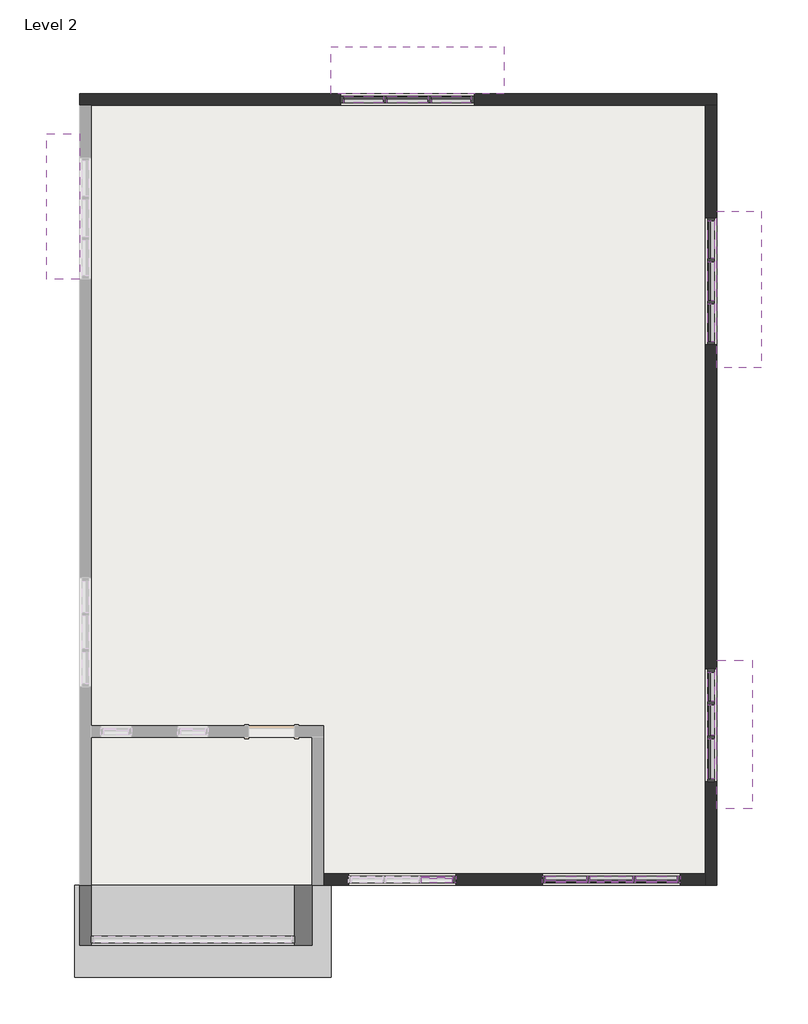
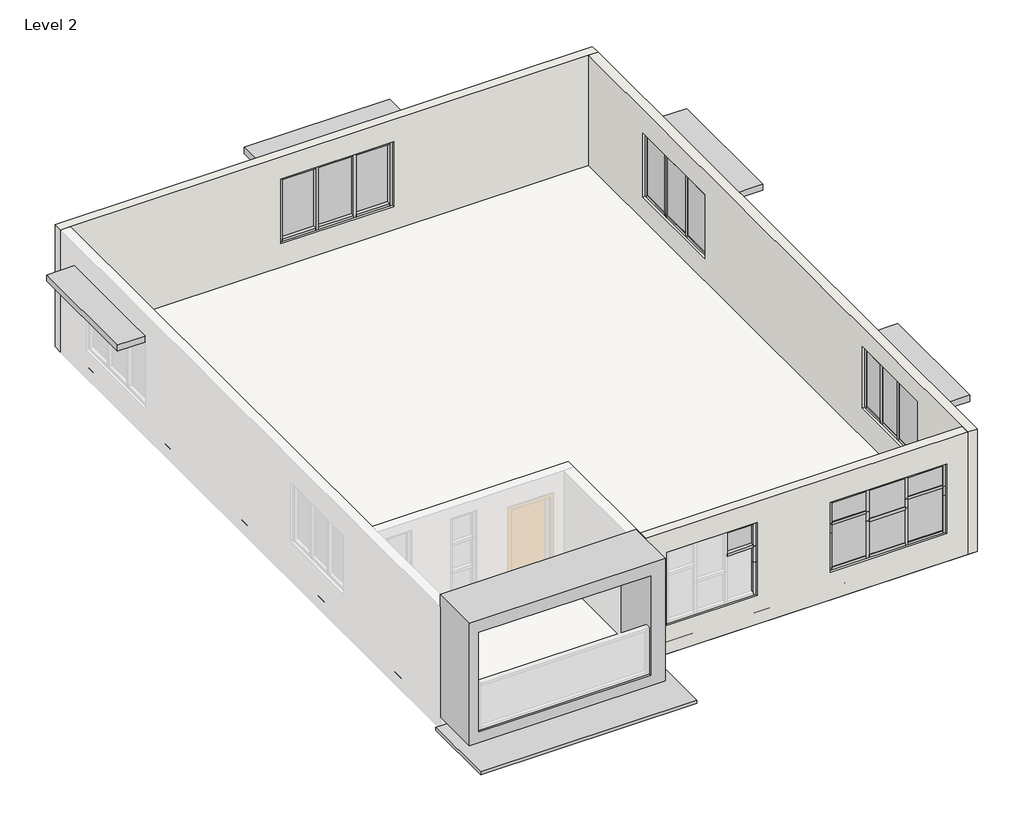
# One storey, part 2 of 2: 56 members, 16 plates, 5 proxies, 3 walls, 1 roof.
"""IFC4 building model written with IfcOpenShell, lengths in millimetres."""

from ifc_helpers import new_model, si_unit, frame, origin, place, context, project, spatial, polyline, outline, extrude, faceted_brep, transform, mapped, element, save
from components import generic_models_11_generic_models_11_762d5f7a, generic_models_12_generic_models_12_d8dec629, generic_models_13_generic_models_13_31af3d75, generic_models_14_generic_models_14_04b71fdd, generic_models_3_generic_models_3_08b937b6, member_3f0e0172, member_f8dc38bf, member_c17f1be2, member_e6e30476, member_4b1d6a2e, member_ad567e07, member_120d0cb6, member_af2dc76d, member_b990fc36, member_f098b74a, member_d2e7e466, member_7db1855a, member_25d88653, member_13f6f031, member_1f059faf, member_67fa2ece, member_13dc6413, member_9b8460a0, member_0e7b3f94, member_29542bbd, member_53377e5f, member_da260789, member_cda0aa81, member_8d789d2e, member_eb0d2563, member_c508cede, member_2d77dfc0, member_8dd5f4d9, system_panel_glazed_48fb4df7, system_panel_glazed_5d767005, system_panel_glazed_d6f3e944, system_panel_glazed_ec316f56, system_panel_glazed_03a03fc4, system_panel_glazed_53576031, system_panel_glazed_db10fc3c, system_panel_glazed_e283e605, system_panel_glazed_230baa0e, system_panel_glazed_33e8df04, system_panel_glazed_7e5766a3, system_panel_glazed_b88d7f0a

model = new_model("IFC4")

# Units and contexts
model_context = context("Model", 3, world=origin())
ifc_project = project(units=[si_unit("LENGTHUNIT", "METRE", prefix="MILLI")], contexts=[model_context])

# Site, building, storey
site = spatial("IfcSite", under=ifc_project)
building = spatial("IfcBuilding", under=site)
storey = spatial("IfcBuildingStorey", under=building, Name="Level 2", Elevation=3048.0)

# Proxies
placement = place(None, origin())
generic_models_11_generic_models_11_shape = generic_models_11_generic_models_11_762d5f7a(model_context)
element("IfcBuildingElementProxy", 1, Name="Generic Models 11 : Generic Models 11", ObjectType="Generic Models 11 : Generic Models 11", at=placement, inside=storey, context=model_context, shape_type="MappedRepresentation", body=[
    mapped(generic_models_11_generic_models_11_shape, transform((0.0, 0.0, 0.0), x_axis=(1.0, 0.0, 0.0), y_axis=(0.0, 1.0, 0.0), z_axis=(0.0, 0.0, 1.0))),
])
generic_models_12_generic_models_12_shape = generic_models_12_generic_models_12_d8dec629(model_context)
element("IfcBuildingElementProxy", 2, Name="Generic Models 12 : Generic Models 12", ObjectType="Generic Models 12 : Generic Models 12", at=placement, inside=storey, context=model_context, shape_type="MappedRepresentation", body=[
    mapped(generic_models_12_generic_models_12_shape, transform((0.0, 0.0, 0.0), x_axis=(1.0, 0.0, 0.0), y_axis=(0.0, 1.0, 0.0), z_axis=(0.0, 0.0, 1.0))),
])
generic_models_13_generic_models_13_shape = generic_models_13_generic_models_13_31af3d75(model_context)
element("IfcBuildingElementProxy", 3, Name="Generic Models 13 : Generic Models 13", ObjectType="Generic Models 13 : Generic Models 13", at=placement, inside=storey, context=model_context, shape_type="MappedRepresentation", body=[
    mapped(generic_models_13_generic_models_13_shape, transform((0.0, 0.0, 0.0), x_axis=(1.0, 0.0, 0.0), y_axis=(0.0, 1.0, 0.0), z_axis=(0.0, 0.0, 1.0))),
])
generic_models_14_generic_models_14_shape = generic_models_14_generic_models_14_04b71fdd(model_context)
element("IfcBuildingElementProxy", 4, Name="Generic Models 14 : Generic Models 14", ObjectType="Generic Models 14 : Generic Models 14", at=placement, inside=storey, context=model_context, shape_type="MappedRepresentation", body=[
    mapped(generic_models_14_generic_models_14_shape, transform((0.0, 0.0, 0.0), x_axis=(1.0, 0.0, 0.0), y_axis=(0.0, 1.0, 0.0), z_axis=(0.0, 0.0, 1.0))),
])
generic_models_3_generic_models_3_shape = generic_models_3_generic_models_3_08b937b6(model_context)
element("IfcBuildingElementProxy", 5, Name="Generic Models 3 : Generic Models 3", ObjectType="Generic Models 3 : Generic Models 3", at=placement, inside=storey, context=model_context, shape_type="MappedRepresentation", body=[
    mapped(generic_models_3_generic_models_3_shape, transform((0.0, 0.0, 0.0), x_axis=(1.0, 0.0, 0.0), y_axis=(0.0, 1.0, 0.0), z_axis=(0.0, 0.0, 1.0))),
])

# Members
member_shape = member_3f0e0172(model_context)
element("IfcMember", 6, ObjectType="Rectangular Mullion : 2.5\" x 5\" rectangular", at=placement, inside=storey, context=model_context, shape_type="MappedRepresentation", body=[
    mapped(member_shape, transform((-14441.5161422, -14789.9171312, 5583.6799972), x_axis=(0.0, 0.0, 1.0), y_axis=(0.0, -1.0, 0.0), z_axis=(1.0, 0.0, 0.0))),
])
member_2_shape = member_f8dc38bf(model_context)
element("IfcMember", 7, ObjectType="Rectangular Mullion : 2.5\" x 5\" rectangular", at=placement, inside=storey, context=model_context, shape_type="MappedRepresentation", body=[
    mapped(member_2_shape, transform((-14441.5161422, -14789.9171312, 4975.0795001), x_axis=(0.0, 0.0, 1.0), y_axis=(0.0, -1.0, 0.0), z_axis=(1.0, 0.0, 0.0))),
])
member_3_shape = member_c17f1be2(model_context)
element("IfcMember", 8, ObjectType="Rectangular Mullion : 2.5\" x 5\" rectangular", at=placement, inside=storey, context=model_context, shape_type="MappedRepresentation", body=[
    mapped(member_3_shape, transform((-10802.9661422, -14789.9171312, 5472.9747898), x_axis=(0.0, 0.0, 1.0), y_axis=(0.0, 1.0, 0.0), z_axis=(-1.0, 0.0, 0.0))),
])
element("IfcMember", 9, ObjectType="Rectangular Mullion : 2.5\" x 5\" rectangular", at=placement, inside=storey, context=model_context, shape_type="MappedRepresentation", body=[
    mapped(member_3_shape, transform((-12600.0161422, -14789.9171312, 5472.9747898), x_axis=(0.0, 0.0, 1.0), y_axis=(0.0, 1.0, 0.0), z_axis=(-1.0, 0.0, 0.0))),
])
element("IfcMember", 10, ObjectType="Rectangular Mullion : 2.5\" x 5\" rectangular", at=placement, inside=storey, context=model_context, shape_type="MappedRepresentation", body=[
    mapped(member_3_shape, transform((-11780.8661422, -14789.9171312, 3739.0267476), x_axis=(0.0, 0.0, -1.0), y_axis=(0.0, 1.0, 0.0), z_axis=(1.0, 0.0, 0.0))),
])
element("IfcMember", 11, ObjectType="Rectangular Mullion : 2.5\" x 5\" rectangular", at=placement, inside=storey, context=model_context, shape_type="MappedRepresentation", body=[
    mapped(member_3_shape, transform((-9983.8161422, -14789.9171312, 3739.0267476), x_axis=(0.0, 0.0, -1.0), y_axis=(0.0, 1.0, 0.0), z_axis=(1.0, 0.0, 0.0))),
])
member_4_shape = member_e6e30476(model_context)
element("IfcMember", 12, ObjectType="Rectangular Mullion : 2.5\" x 5\" rectangular", at=placement, inside=storey, context=model_context, shape_type="MappedRepresentation", body=[
    mapped(member_4_shape, transform((-12663.5161422, -14789.9171312, 3739.0267476), x_axis=(-1.0, 0.0, 0.0), y_axis=(0.0, 1.0, 0.0), z_axis=(0.0, 0.0, -1.0))),
])
member_5_shape = member_4b1d6a2e(model_context)
element("IfcMember", 13, ObjectType="Rectangular Mullion : 2.5\" x 5\" rectangular", at=placement, inside=storey, context=model_context, shape_type="MappedRepresentation", body=[
    mapped(member_5_shape, transform((-11749.1161422, -14789.9171312, 4894.992109), x_axis=(-1.0, 0.0, 0.0), y_axis=(0.0, 1.0, 0.0), z_axis=(0.0, 0.0, -1.0))),
])
element("IfcMember", 14, ObjectType="Rectangular Mullion : 2.5\" x 5\" rectangular", at=placement, inside=storey, context=model_context, shape_type="MappedRepresentation", body=[
    mapped(member_5_shape, transform((-10834.7161422, -14789.9171312, 4894.992109), x_axis=(-1.0, 0.0, 0.0), y_axis=(0.0, 1.0, 0.0), z_axis=(0.0, 0.0, -1.0))),
])
member_6_shape = member_ad567e07(model_context)
element("IfcMember", 15, ObjectType="Rectangular Mullion : 2.5\" x 5\" rectangular", at=placement, inside=storey, context=model_context, shape_type="MappedRepresentation", body=[
    mapped(member_6_shape, transform((-12600.0161422, -14789.9171312, 4894.992109), x_axis=(0.0, 0.0, 1.0), y_axis=(0.0, 1.0, 0.0), z_axis=(-1.0, 0.0, 0.0))),
])
element("IfcMember", 16, ObjectType="Rectangular Mullion : 2.5\" x 5\" rectangular", at=placement, inside=storey, context=model_context, shape_type="MappedRepresentation", body=[
    mapped(member_6_shape, transform((-10802.9661422, -14789.9171312, 4894.992109), x_axis=(0.0, 0.0, 1.0), y_axis=(0.0, 1.0, 0.0), z_axis=(-1.0, 0.0, 0.0))),
])
member_7_shape = member_120d0cb6(model_context)
element("IfcMember", 17, ObjectType="Rectangular Mullion : 2.5\" x 5\" rectangular", at=placement, inside=storey, context=model_context, shape_type="MappedRepresentation", body=[
    mapped(member_7_shape, transform((-12663.5161422, -14789.9171312, 4666.392109), x_axis=(-1.0, 0.0, 0.0), y_axis=(0.0, 1.0, 0.0), z_axis=(0.0, 0.0, -1.0))),
])
member_8_shape = member_af2dc76d(model_context)
element("IfcMember", 18, ObjectType="Rectangular Mullion : 2.5\" x 5\" rectangular", at=placement, inside=storey, context=model_context, shape_type="MappedRepresentation", body=[
    mapped(member_8_shape, transform((-12663.5161422, -14789.9171312, 4894.992109), x_axis=(-1.0, 0.0, 0.0), y_axis=(0.0, 1.0, 0.0), z_axis=(0.0, 0.0, -1.0))),
])
member_9_shape = member_b990fc36(model_context)
element("IfcMember", 19, ObjectType="Rectangular Mullion : 2.5\" x 5\" rectangular", at=placement, inside=storey, context=model_context, shape_type="MappedRepresentation", body=[
    mapped(member_9_shape, transform((-11749.1161422, -14789.9171312, 4666.392109), x_axis=(-1.0, 0.0, 0.0), y_axis=(0.0, 1.0, 0.0), z_axis=(0.0, 0.0, -1.0))),
])
element("IfcMember", 20, ObjectType="Rectangular Mullion : 2.5\" x 5\" rectangular", at=placement, inside=storey, context=model_context, shape_type="MappedRepresentation", body=[
    mapped(member_9_shape, transform((-10834.7161422, -14789.9171312, 4666.392109), x_axis=(-1.0, 0.0, 0.0), y_axis=(0.0, 1.0, 0.0), z_axis=(0.0, 0.0, -1.0))),
])
member_10_shape = member_f098b74a(model_context)
element("IfcMember", 21, ObjectType="Rectangular Mullion : 2.5\" x 5\" rectangular", at=placement, inside=storey, context=model_context, shape_type="MappedRepresentation", body=[
    mapped(member_10_shape, transform((-11749.1161422, -14789.9171312, 3739.0267476), x_axis=(-1.0, 0.0, 0.0), y_axis=(0.0, 1.0, 0.0), z_axis=(0.0, 0.0, -1.0))),
])
element("IfcMember", 22, ObjectType="Rectangular Mullion : 2.5\" x 5\" rectangular", at=placement, inside=storey, context=model_context, shape_type="MappedRepresentation", body=[
    mapped(member_10_shape, transform((-10834.7161422, -14789.9171312, 3739.0267476), x_axis=(-1.0, 0.0, 0.0), y_axis=(0.0, 1.0, 0.0), z_axis=(0.0, 0.0, -1.0))),
])
member_11_shape = member_d2e7e466(model_context)
element("IfcMember", 23, ObjectType="Rectangular Mullion : 2.5\" x 5\" rectangular", at=placement, inside=storey, context=model_context, shape_type="MappedRepresentation", body=[
    mapped(member_11_shape, transform((-11717.3661422, -14789.9171312, 5472.9747898), x_axis=(0.0, 0.0, 1.0), y_axis=(0.0, 1.0, 0.0), z_axis=(-1.0, 0.0, 0.0))),
])
element("IfcMember", 24, ObjectType="Rectangular Mullion : 2.5\" x 5\" rectangular", at=placement, inside=storey, context=model_context, shape_type="MappedRepresentation", body=[
    mapped(member_11_shape, transform((-10866.4661422, -14789.9171312, 3739.0267476), x_axis=(0.0, 0.0, -1.0), y_axis=(0.0, 1.0, 0.0), z_axis=(1.0, 0.0, 0.0))),
])
member_12_shape = member_7db1855a(model_context)
element("IfcMember", 25, ObjectType="Rectangular Mullion : 2.5\" x 5\" rectangular", at=placement, inside=storey, context=model_context, shape_type="MappedRepresentation", body=[
    mapped(member_12_shape, transform((-11717.3661422, -14789.9171312, 4666.392109), x_axis=(0.0, 0.0, 1.0), y_axis=(0.0, 1.0, 0.0), z_axis=(-1.0, 0.0, 0.0))),
])
element("IfcMember", 26, ObjectType="Rectangular Mullion : 2.5\" x 5\" rectangular", at=placement, inside=storey, context=model_context, shape_type="MappedRepresentation", body=[
    mapped(member_4_shape, transform((-9920.3161422, -14789.9171312, 4666.392109), x_axis=(1.0, 0.0, 0.0), y_axis=(0.0, 1.0, 0.0), z_axis=(0.0, 0.0, 1.0))),
])
element("IfcMember", 27, ObjectType="Rectangular Mullion : 2.5\" x 5\" rectangular", at=placement, inside=storey, context=model_context, shape_type="MappedRepresentation", body=[
    mapped(member_7_shape, transform((-9920.3161422, -14789.9171312, 4894.992109), x_axis=(1.0, 0.0, 0.0), y_axis=(0.0, 1.0, 0.0), z_axis=(0.0, 0.0, 1.0))),
])
element("IfcMember", 28, ObjectType="Rectangular Mullion : 2.5\" x 5\" rectangular", at=placement, inside=storey, context=model_context, shape_type="MappedRepresentation", body=[
    mapped(member_8_shape, transform((-9920.3161422, -14789.9171312, 5472.9747898), x_axis=(1.0, 0.0, 0.0), y_axis=(0.0, 1.0, 0.0), z_axis=(0.0, 0.0, 1.0))),
])
member_13_shape = member_25d88653(model_context)
element("IfcMember", 29, ObjectType="Rectangular Mullion : 2.5\" x 5\" rectangular", at=placement, inside=storey, context=model_context, shape_type="MappedRepresentation", body=[
    mapped(member_13_shape, transform((-14378.0161422, -14789.9171312, 4569.3458353), x_axis=(1.0, 0.0, 0.0), y_axis=(0.0, -1.0, 0.0), z_axis=(0.0, 0.0, -1.0))),
])
member_14_shape = member_13f6f031(model_context)
element("IfcMember", 30, ObjectType="Rectangular Mullion : 2.5\" x 5\" rectangular", at=placement, inside=storey, context=model_context, shape_type="MappedRepresentation", body=[
    mapped(member_14_shape, transform((-14378.0161422, -14789.9171312, 4975.0795001), x_axis=(1.0, 0.0, 0.0), y_axis=(0.0, -1.0, 0.0), z_axis=(0.0, 0.0, -1.0))),
])
member_15_shape = member_1f059faf(model_context)
element("IfcMember", 31, ObjectType="Rectangular Mullion : 2.5\" x 5\" rectangular", at=placement, inside=storey, context=model_context, shape_type="MappedRepresentation", body=[
    mapped(member_15_shape, transform((-14378.0161422, -14789.9171312, 3757.8785057), x_axis=(1.0, 0.0, 0.0), y_axis=(0.0, -1.0, 0.0), z_axis=(0.0, 0.0, -1.0))),
])
member_16_shape = member_67fa2ece(model_context)
element("IfcMember", 32, ObjectType="Rectangular Mullion : 2.5\" x 5\" rectangular", at=placement, inside=storey, context=model_context, shape_type="MappedRepresentation", body=[
    mapped(member_16_shape, transform((-9310.7161422, -11320.6000267, 5616.1380633), x_axis=(0.0, 0.0, 1.0), y_axis=(1.0, 0.0, 0.0), z_axis=(0.0, 1.0, 0.0))),
])
member_17_shape = member_13dc6413(model_context)
element("IfcMember", 33, ObjectType="Rectangular Mullion : 2.5\" x 5\" rectangular", at=placement, inside=storey, context=model_context, shape_type="MappedRepresentation", body=[
    mapped(member_17_shape, transform((-9310.7161422, -11997.8329222, 5616.1380633), x_axis=(0.0, 0.0, 1.0), y_axis=(1.0, 0.0, 0.0), z_axis=(0.0, 1.0, 0.0))),
])
member_18_shape = member_9b8460a0(model_context)
element("IfcMember", 34, ObjectType="Rectangular Mullion : 2.5\" x 5\" rectangular", at=placement, inside=storey, context=model_context, shape_type="MappedRepresentation", body=[
    mapped(member_18_shape, transform((-9310.7161422, -10675.1171312, 5616.1380633), x_axis=(0.0, 0.0, 1.0), y_axis=(1.0, 0.0, 0.0), z_axis=(0.0, 1.0, 0.0))),
])
member_19_shape = member_0e7b3f94(model_context)
element("IfcMember", 35, ObjectType="Rectangular Mullion : 2.5\" x 5\" rectangular", at=placement, inside=storey, context=model_context, shape_type="MappedRepresentation", body=[
    mapped(member_19_shape, transform((-9310.7161422, -11966.0829222, 4087.473097), x_axis=(0.0, 1.0, 0.0), y_axis=(1.0, 0.0, 0.0), z_axis=(0.0, 0.0, -1.0))),
])
element("IfcMember", 36, ObjectType="Rectangular Mullion : 2.5\" x 5\" rectangular", at=placement, inside=storey, context=model_context, shape_type="MappedRepresentation", body=[
    mapped(member_19_shape, transform((-9310.7161422, -11288.8500267, 4087.473097), x_axis=(0.0, 1.0, 0.0), y_axis=(1.0, 0.0, 0.0), z_axis=(0.0, 0.0, -1.0))),
])
element("IfcMember", 37, ObjectType="Rectangular Mullion : 2.5\" x 5\" rectangular", at=placement, inside=storey, context=model_context, shape_type="MappedRepresentation", body=[
    mapped(member_18_shape, transform((-9310.7161422, -11257.1000267, 4087.473097), x_axis=(0.0, 0.0, -1.0), y_axis=(1.0, 0.0, 0.0), z_axis=(0.0, -1.0, 0.0))),
])
element("IfcMember", 38, ObjectType="Rectangular Mullion : 2.5\" x 5\" rectangular", at=placement, inside=storey, context=model_context, shape_type="MappedRepresentation", body=[
    mapped(member_16_shape, transform((-9310.7161422, -11934.3329222, 4087.473097), x_axis=(0.0, 0.0, -1.0), y_axis=(1.0, 0.0, 0.0), z_axis=(0.0, -1.0, 0.0))),
])
element("IfcMember", 39, ObjectType="Rectangular Mullion : 2.5\" x 5\" rectangular", at=placement, inside=storey, context=model_context, shape_type="MappedRepresentation", body=[
    mapped(member_17_shape, transform((-9310.7161422, -12791.5829222, 4087.473097), x_axis=(0.0, 0.0, -1.0), y_axis=(1.0, 0.0, 0.0), z_axis=(0.0, -1.0, 0.0))),
])
member_20_shape = member_29542bbd(model_context)
element("IfcMember", 40, ObjectType="Rectangular Mullion : 2.5\" x 5\" rectangular", at=placement, inside=storey, context=model_context, shape_type="MappedRepresentation", body=[
    mapped(member_20_shape, transform((-9310.7161422, -10611.6171312, 4087.473097), x_axis=(0.0, 1.0, 0.0), y_axis=(1.0, 0.0, 0.0), z_axis=(0.0, 0.0, -1.0))),
])
element("IfcMember", 41, ObjectType="Rectangular Mullion : 2.5\" x 5\" rectangular", at=placement, inside=storey, context=model_context, shape_type="MappedRepresentation", body=[
    mapped(member_20_shape, transform((-9310.7161422, -12855.0829222, 5616.1380633), x_axis=(0.0, -1.0, 0.0), y_axis=(1.0, 0.0, 0.0), z_axis=(0.0, 0.0, 1.0))),
])
member_21_shape = member_53377e5f(model_context)
element("IfcMember", 42, ObjectType="Rectangular Mullion : 2.5\" x 5\" rectangular", at=placement, inside=storey, context=model_context, shape_type="MappedRepresentation", body=[
    mapped(member_21_shape, transform((-9310.7161422, -2533.2020504, 5503.6617435), x_axis=(0.0, 0.0, 1.0), y_axis=(1.0, 0.0, 0.0), z_axis=(0.0, 1.0, 0.0))),
])
member_22_shape = member_da260789(model_context)
element("IfcMember", 43, ObjectType="Rectangular Mullion : 2.5\" x 5\" rectangular", at=placement, inside=storey, context=model_context, shape_type="MappedRepresentation", body=[
    mapped(member_22_shape, transform((-9310.7161422, -3373.9897607, 5503.6617435), x_axis=(0.0, 0.0, 1.0), y_axis=(1.0, 0.0, 0.0), z_axis=(0.0, 1.0, 0.0))),
])
element("IfcMember", 44, ObjectType="Rectangular Mullion : 2.5\" x 5\" rectangular", at=placement, inside=storey, context=model_context, shape_type="MappedRepresentation", body=[
    mapped(member_22_shape, transform((-9310.7161422, -1724.1643401, 5503.6617435), x_axis=(0.0, 0.0, 1.0), y_axis=(1.0, 0.0, 0.0), z_axis=(0.0, 1.0, 0.0))),
])
member_23_shape = member_cda0aa81(model_context)
element("IfcMember", 45, ObjectType="Rectangular Mullion : 2.5\" x 5\" rectangular", at=placement, inside=storey, context=model_context, shape_type="MappedRepresentation", body=[
    mapped(member_23_shape, transform((-9310.7161422, -3342.2397607, 3916.1325572), x_axis=(0.0, 1.0, 0.0), y_axis=(1.0, 0.0, 0.0), z_axis=(0.0, 0.0, -1.0))),
])
element("IfcMember", 46, ObjectType="Rectangular Mullion : 2.5\" x 5\" rectangular", at=placement, inside=storey, context=model_context, shape_type="MappedRepresentation", body=[
    mapped(member_23_shape, transform((-9310.7161422, -2501.4520504, 3916.1325572), x_axis=(0.0, 1.0, 0.0), y_axis=(1.0, 0.0, 0.0), z_axis=(0.0, 0.0, -1.0))),
])
element("IfcMember", 47, ObjectType="Rectangular Mullion : 2.5\" x 5\" rectangular", at=placement, inside=storey, context=model_context, shape_type="MappedRepresentation", body=[
    mapped(member_22_shape, transform((-9310.7161422, -2469.7020504, 3916.1325572), x_axis=(0.0, 0.0, -1.0), y_axis=(1.0, 0.0, 0.0), z_axis=(0.0, -1.0, 0.0))),
])
element("IfcMember", 48, ObjectType="Rectangular Mullion : 2.5\" x 5\" rectangular", at=placement, inside=storey, context=model_context, shape_type="MappedRepresentation", body=[
    mapped(member_22_shape, transform((-9310.7161422, -4119.527471, 3916.1325572), x_axis=(0.0, 0.0, -1.0), y_axis=(1.0, 0.0, 0.0), z_axis=(0.0, -1.0, 0.0))),
])
element("IfcMember", 49, ObjectType="Rectangular Mullion : 2.5\" x 5\" rectangular", at=placement, inside=storey, context=model_context, shape_type="MappedRepresentation", body=[
    mapped(member_21_shape, transform((-9310.7161422, -3310.4897607, 3916.1325572), x_axis=(0.0, 0.0, -1.0), y_axis=(1.0, 0.0, 0.0), z_axis=(0.0, -1.0, 0.0))),
])
member_24_shape = member_8d789d2e(model_context)
element("IfcMember", 50, ObjectType="Rectangular Mullion : 2.5\" x 5\" rectangular", at=placement, inside=storey, context=model_context, shape_type="MappedRepresentation", body=[
    mapped(member_24_shape, transform((-9310.7161422, -1660.6643401, 3916.1325572), x_axis=(0.0, 1.0, 0.0), y_axis=(1.0, 0.0, 0.0), z_axis=(0.0, 0.0, -1.0))),
])
element("IfcMember", 51, ObjectType="Rectangular Mullion : 2.5\" x 5\" rectangular", at=placement, inside=storey, context=model_context, shape_type="MappedRepresentation", body=[
    mapped(member_24_shape, transform((-9310.7161422, -4183.027471, 5503.6617435), x_axis=(0.0, -1.0, 0.0), y_axis=(1.0, 0.0, 0.0), z_axis=(0.0, 0.0, 1.0))),
])
member_25_shape = member_eb0d2563(model_context)
element("IfcMember", 52, ObjectType="Rectangular Mullion : 2.5\" x 5\" rectangular", at=placement, inside=storey, context=model_context, shape_type="MappedRepresentation", body=[
    mapped(member_25_shape, transform((-14926.7023392, 678.6828688, 5544.590558), x_axis=(0.0, 0.0, 1.0), y_axis=(0.0, -1.0, 0.0), z_axis=(1.0, 0.0, 0.0))),
])
member_26_shape = member_c508cede(model_context)
element("IfcMember", 53, ObjectType="Rectangular Mullion : 2.5\" x 5\" rectangular", at=placement, inside=storey, context=model_context, shape_type="MappedRepresentation", body=[
    mapped(member_26_shape, transform((-15811.9385362, 678.6828688, 5544.590558), x_axis=(0.0, 0.0, 1.0), y_axis=(0.0, -1.0, 0.0), z_axis=(1.0, 0.0, 0.0))),
])
element("IfcMember", 54, ObjectType="Rectangular Mullion : 2.5\" x 5\" rectangular", at=placement, inside=storey, context=model_context, shape_type="MappedRepresentation", body=[
    mapped(member_26_shape, transform((-14073.2161422, 678.6828688, 5544.590558), x_axis=(0.0, 0.0, 1.0), y_axis=(0.0, -1.0, 0.0), z_axis=(1.0, 0.0, 0.0))),
])
member_27_shape = member_2d77dfc0(model_context)
element("IfcMember", 55, ObjectType="Rectangular Mullion : 2.5\" x 5\" rectangular", at=placement, inside=storey, context=model_context, shape_type="MappedRepresentation", body=[
    mapped(member_27_shape, transform((-14894.9523392, 678.6828688, 3939.0070554), x_axis=(1.0, 0.0, 0.0), y_axis=(0.0, -1.0, 0.0), z_axis=(0.0, 0.0, -1.0))),
])
element("IfcMember", 56, ObjectType="Rectangular Mullion : 2.5\" x 5\" rectangular", at=placement, inside=storey, context=model_context, shape_type="MappedRepresentation", body=[
    mapped(member_27_shape, transform((-15780.1885362, 678.6828688, 3939.0070554), x_axis=(1.0, 0.0, 0.0), y_axis=(0.0, -1.0, 0.0), z_axis=(0.0, 0.0, -1.0))),
])
element("IfcMember", 57, ObjectType="Rectangular Mullion : 2.5\" x 5\" rectangular", at=placement, inside=storey, context=model_context, shape_type="MappedRepresentation", body=[
    mapped(member_25_shape, transform((-15748.4385362, 678.6828688, 3939.0070554), x_axis=(0.0, 0.0, -1.0), y_axis=(0.0, -1.0, 0.0), z_axis=(-1.0, 0.0, 0.0))),
])
element("IfcMember", 58, ObjectType="Rectangular Mullion : 2.5\" x 5\" rectangular", at=placement, inside=storey, context=model_context, shape_type="MappedRepresentation", body=[
    mapped(member_26_shape, transform((-14863.2023392, 678.6828688, 3939.0070554), x_axis=(0.0, 0.0, -1.0), y_axis=(0.0, -1.0, 0.0), z_axis=(-1.0, 0.0, 0.0))),
])
element("IfcMember", 59, ObjectType="Rectangular Mullion : 2.5\" x 5\" rectangular", at=placement, inside=storey, context=model_context, shape_type="MappedRepresentation", body=[
    mapped(member_26_shape, transform((-16601.9247332, 678.6828688, 3939.0070554), x_axis=(0.0, 0.0, -1.0), y_axis=(0.0, -1.0, 0.0), z_axis=(-1.0, 0.0, 0.0))),
])
member_28_shape = member_8dd5f4d9(model_context)
element("IfcMember", 60, ObjectType="Rectangular Mullion : 2.5\" x 5\" rectangular", at=placement, inside=storey, context=model_context, shape_type="MappedRepresentation", body=[
    mapped(member_28_shape, transform((-14009.7161422, 678.6828688, 3939.0070554), x_axis=(1.0, 0.0, 0.0), y_axis=(0.0, -1.0, 0.0), z_axis=(0.0, 0.0, -1.0))),
])
element("IfcMember", 61, ObjectType="Rectangular Mullion : 2.5\" x 5\" rectangular", at=placement, inside=storey, context=model_context, shape_type="MappedRepresentation", body=[
    mapped(member_28_shape, transform((-16665.4247332, 678.6828688, 5544.590558), x_axis=(-1.0, 0.0, 0.0), y_axis=(0.0, -1.0, 0.0), z_axis=(0.0, 0.0, 1.0))),
])

# Plates
system_panel_glazed_shape = system_panel_glazed_48fb4df7(model_context)
element("IfcPlate", 62, ObjectType="System Panel : Glazed", at=placement, inside=storey, context=model_context, shape_type="MappedRepresentation", body=[
    mapped(system_panel_glazed_shape, transform((-10393.3911422, -14789.9171312, 3802.5267476), x_axis=(-1.0, 0.0, 0.0), y_axis=(0.0, -1.0, 0.0), z_axis=(0.0, 0.0, 1.0))),
])
element("IfcPlate", 63, ObjectType="System Panel : Glazed", at=placement, inside=storey, context=model_context, shape_type="MappedRepresentation", body=[
    mapped(system_panel_glazed_shape, transform((-12190.4411422, -14789.9171312, 3802.5267476), x_axis=(-1.0, 0.0, 0.0), y_axis=(0.0, -1.0, 0.0), z_axis=(0.0, 0.0, 1.0))),
])
system_panel_glazed_2_shape = system_panel_glazed_5d767005(model_context)
element("IfcPlate", 64, ObjectType="System Panel : Glazed", at=placement, inside=storey, context=model_context, shape_type="MappedRepresentation", body=[
    mapped(system_panel_glazed_2_shape, transform((-10393.3911422, -14789.9171312, 4926.742109), x_axis=(-1.0, 0.0, 0.0), y_axis=(0.0, -1.0, 0.0), z_axis=(0.0, 0.0, 1.0))),
])
element("IfcPlate", 65, ObjectType="System Panel : Glazed", at=placement, inside=storey, context=model_context, shape_type="MappedRepresentation", body=[
    mapped(system_panel_glazed_2_shape, transform((-12190.4411422, -14789.9171312, 4926.742109), x_axis=(-1.0, 0.0, 0.0), y_axis=(0.0, -1.0, 0.0), z_axis=(0.0, 0.0, 1.0))),
])
system_panel_glazed_3_shape = system_panel_glazed_d6f3e944(model_context)
element("IfcPlate", 66, ObjectType="System Panel : Glazed", at=placement, inside=storey, context=model_context, shape_type="MappedRepresentation", body=[
    mapped(system_panel_glazed_3_shape, transform((-11291.9161422, -14789.9171312, 3802.5267476), x_axis=(-1.0, 0.0, 0.0), y_axis=(0.0, -1.0, 0.0), z_axis=(0.0, 0.0, 1.0))),
])
system_panel_glazed_4_shape = system_panel_glazed_ec316f56(model_context)
element("IfcPlate", 67, ObjectType="System Panel : Glazed", at=placement, inside=storey, context=model_context, shape_type="MappedRepresentation", body=[
    mapped(system_panel_glazed_4_shape, transform((-11291.9161422, -14789.9171312, 4698.142109), x_axis=(-1.0, 0.0, 0.0), y_axis=(0.0, -1.0, 0.0), z_axis=(0.0, 0.0, 1.0))),
])
system_panel_glazed_5_shape = system_panel_glazed_03a03fc4(model_context)
element("IfcPlate", 68, ObjectType="System Panel : Glazed", at=placement, inside=storey, context=model_context, shape_type="MappedRepresentation", body=[
    mapped(system_panel_glazed_5_shape, transform((-14749.4911422, -14789.9171312, 5006.8295001), x_axis=(1.0, 0.0, 0.0), y_axis=(0.0, 1.0, 0.0), z_axis=(0.0, 0.0, 1.0))),
])
system_panel_glazed_6_shape = system_panel_glazed_53576031(model_context)
element("IfcPlate", 69, ObjectType="System Panel : Glazed", at=placement, inside=storey, context=model_context, shape_type="MappedRepresentation", body=[
    mapped(system_panel_glazed_6_shape, transform((-9310.7161422, -12394.7079222, 4150.973097), x_axis=(0.0, 1.0, 0.0), y_axis=(-1.0, 0.0, 0.0), z_axis=(0.0, 0.0, 1.0))),
])
system_panel_glazed_7_shape = system_panel_glazed_db10fc3c(model_context)
element("IfcPlate", 70, ObjectType="System Panel : Glazed", at=placement, inside=storey, context=model_context, shape_type="MappedRepresentation", body=[
    mapped(system_panel_glazed_7_shape, transform((-9310.7161422, -11627.4664744, 4150.973097), x_axis=(0.0, 1.0, 0.0), y_axis=(-1.0, 0.0, 0.0), z_axis=(0.0, 0.0, 1.0))),
])
system_panel_glazed_8_shape = system_panel_glazed_e283e605(model_context)
element("IfcPlate", 71, ObjectType="System Panel : Glazed", at=placement, inside=storey, context=model_context, shape_type="MappedRepresentation", body=[
    mapped(system_panel_glazed_8_shape, transform((-9310.7161422, -10966.108579, 4150.973097), x_axis=(0.0, 1.0, 0.0), y_axis=(-1.0, 0.0, 0.0), z_axis=(0.0, 0.0, 1.0))),
])
system_panel_glazed_9_shape = system_panel_glazed_230baa0e(model_context)
element("IfcPlate", 72, ObjectType="System Panel : Glazed", at=placement, inside=storey, context=model_context, shape_type="MappedRepresentation", body=[
    mapped(system_panel_glazed_9_shape, transform((-9310.7161422, -3746.7586159, 3979.6325572), x_axis=(0.0, 1.0, 0.0), y_axis=(-1.0, 0.0, 0.0), z_axis=(0.0, 0.0, 1.0))),
])
element("IfcPlate", 73, ObjectType="System Panel : Glazed", at=placement, inside=storey, context=model_context, shape_type="MappedRepresentation", body=[
    mapped(system_panel_glazed_9_shape, transform((-9310.7161422, -2096.9331953, 3979.6325572), x_axis=(0.0, 1.0, 0.0), y_axis=(-1.0, 0.0, 0.0), z_axis=(0.0, 0.0, 1.0))),
])
system_panel_glazed_10_shape = system_panel_glazed_33e8df04(model_context)
element("IfcPlate", 74, ObjectType="System Panel : Glazed", at=placement, inside=storey, context=model_context, shape_type="MappedRepresentation", body=[
    mapped(system_panel_glazed_10_shape, transform((-9310.7161422, -2921.8459056, 3979.6325572), x_axis=(0.0, 1.0, 0.0), y_axis=(-1.0, 0.0, 0.0), z_axis=(0.0, 0.0, 1.0))),
])
system_panel_glazed_11_shape = system_panel_glazed_7e5766a3(model_context)
element("IfcPlate", 75, ObjectType="System Panel : Glazed", at=placement, inside=storey, context=model_context, shape_type="MappedRepresentation", body=[
    mapped(system_panel_glazed_11_shape, transform((-16206.9316347, 678.6828688, 4002.5070554), x_axis=(1.0, 0.0, 0.0), y_axis=(0.0, 1.0, 0.0), z_axis=(0.0, 0.0, 1.0))),
])
element("IfcPlate", 76, ObjectType="System Panel : Glazed", at=placement, inside=storey, context=model_context, shape_type="MappedRepresentation", body=[
    mapped(system_panel_glazed_11_shape, transform((-14468.2092407, 678.6828688, 4002.5070554), x_axis=(1.0, 0.0, 0.0), y_axis=(0.0, 1.0, 0.0), z_axis=(0.0, 0.0, 1.0))),
])
system_panel_glazed_12_shape = system_panel_glazed_b88d7f0a(model_context)
element("IfcPlate", 77, ObjectType="System Panel : Glazed", at=placement, inside=storey, context=model_context, shape_type="MappedRepresentation", body=[
    mapped(system_panel_glazed_12_shape, transform((-15337.5704377, 678.6828688, 4002.5070554), x_axis=(1.0, 0.0, 0.0), y_axis=(0.0, 1.0, 0.0), z_axis=(0.0, 0.0, 1.0))),
])

# Roof
element("IfcRoof", 78, ObjectType="Generic - 12\"", at=placement, inside=storey, context=model_context, shape_type="SweptSolid", body=[
    extrude(outline(polyline([(-21845.6161422, 792.9828688), (-9196.4161422, 792.9828688), (-9196.4161422, -14904.2171312), (-21845.6161422, -14904.2171312), (-21845.6161422, 792.9828688)])), frame((0.0, 0.0, 3048.0), z_axis=(0.0, 0.0, 1.0), x_axis=(1.0, 0.0, 0.0)), (0.0, 0.0, 1.0), 304.8),
])

# Walls
element("IfcWall", 79, ObjectType="9\"", at=placement, inside=storey, context=model_context, shape_type="Brep", body=[
    faceted_brep([(-21845.6161422, 564.3828688, 3048.0), (-21617.0161422, 564.3828688, 3048.0), (-9425.0161422, 564.3828688, 3048.0), (-9196.4161422, 564.3828688, 3048.0), (-9196.4161422, 564.3828688, 6096.0), (-9425.0161422, 564.3828688, 6096.0), (-21617.0161422, 564.3828688, 6096.0), (-21845.6161422, 564.3828688, 6096.0), (-16665.4247332, 564.3828688, 3939.0070554), (-16665.4247332, 564.3828688, 5544.590558), (-14009.7161422, 564.3828688, 5544.590558), (-14009.7161422, 564.3828688, 3939.0070554), (-9196.4161422, 792.9828688, 3048.0), (-21845.6161422, 792.9828688, 3048.0), (-21845.6161422, 792.9828688, 6096.0), (-9196.4161422, 792.9828688, 6096.0), (-16665.4247332, 792.9828688, 5544.590558), (-16665.4247332, 792.9828688, 3939.0070554), (-14009.7161422, 792.9828688, 3939.0070554), (-14009.7161422, 792.9828688, 5544.590558)], [[[0, 1, 2, 3, 4, 5, 6, 7], [8, 9, 10, 11]], [[12, 13, 14, 15], [16, 17, 18, 19]], [[3, 2, 1, 0, 13, 12]], [[7, 6, 5, 4, 15, 14]], [[4, 3, 12, 15]], [[0, 7, 14, 13]], [[8, 17, 16, 9]], [[9, 16, 19, 10]], [[10, 19, 18, 11]], [[17, 8, 11, 18]]]),
])
element("IfcWall", 80, ObjectType="9\"", at=placement, inside=storey, context=model_context, shape_type="Brep", body=[
    faceted_brep([(-9425.0161422, 564.3828688, 3048.0), (-9425.0161422, -14675.6171312, 3048.0), (-9425.0161422, -14904.2171312, 3048.0), (-9425.0161422, -14904.2171312, 6096.0), (-9425.0161422, -14675.6171312, 6096.0), (-9425.0161422, 564.3828688, 6096.0), (-9425.0161422, -12855.0829222, 5616.1380633), (-9425.0161422, -12855.0829222, 4087.473097), (-9425.0161422, -10611.6171312, 4087.473097), (-9425.0161422, -10611.6171312, 5616.1380633), (-9425.0161422, -4183.027471, 5503.6617435), (-9425.0161422, -4183.027471, 3916.1325572), (-9425.0161422, -1660.6643401, 3916.1325572), (-9425.0161422, -1660.6643401, 5503.6617435), (-9196.4161422, -14904.2171312, 3048.0), (-9196.4161422, 564.3828688, 3048.0), (-9196.4161422, 564.3828688, 6096.0), (-9196.4161422, -14904.2171312, 6096.0), (-9196.4161422, -12855.0829222, 4087.473097), (-9196.4161422, -12855.0829222, 5616.1380633), (-9196.4161422, -10611.6171312, 5616.1380633), (-9196.4161422, -10611.6171312, 4087.473097), (-9196.4161422, -4183.027471, 3916.1325572), (-9196.4161422, -4183.027471, 5503.6617435), (-9196.4161422, -1660.6643401, 5503.6617435), (-9196.4161422, -1660.6643401, 3916.1325572)], [[[0, 1, 2, 3, 4, 5], [6, 7, 8, 9], [10, 11, 12, 13]], [[14, 15, 16, 17], [18, 19, 20, 21], [22, 23, 24, 25]], [[2, 1, 0, 15, 14]], [[5, 4, 3, 17, 16]], [[0, 5, 16, 15]], [[3, 2, 14, 17]], [[6, 19, 18, 7]], [[19, 6, 9, 20]], [[20, 9, 8, 21]], [[7, 18, 21, 8]], [[22, 11, 10, 23]], [[23, 10, 13, 24]], [[24, 13, 12, 25]], [[11, 22, 25, 12]]]),
])
element("IfcWall", 81, ObjectType="9\"", at=placement, inside=storey, context=model_context, shape_type="SweptSolid", body=[
    extrude(outline(polyline([(3048.0, -17006.9161422), (3048.0, -9425.0161422), (6096.0, -9425.0161422), (6096.0, -17006.9161422), (3048.0, -17006.9161422)]), holes=[polyline([(3757.8785057, -16511.6161422), (5583.6799972, -16511.6161422), (5583.6799972, -14378.0161422), (3757.8785057, -14378.0161422), (3757.8785057, -16511.6161422)]), polyline([(5472.9747898, -9920.3161422), (3739.0267476, -9920.3161422), (3739.0267476, -12663.5161422), (5472.9747898, -12663.5161422), (5472.9747898, -9920.3161422)])]), frame((0.0, -14904.2171312, 0.0), z_axis=(0.0, 1.0, 0.0), x_axis=(0.0, 0.0, 1.0)), (0.0, 0.0, 1.0), 228.6),
])

save(model, "model.ifc")

# Revit data of these elements
# Type "Rectangular Mullion : 2.5\" x 5\" rectangular"
#   built-in parameter 1007304 = 0.416667 (stored number, unit not read)
#   built-in parameter 1007301 = 0.104167 (stored number, unit not read)
#   built-in parameter 1007300 = 0.104167 (stored number, unit not read)
# Type "System Panel : Glazed"
#   Construction Type Id = "GSP4R"
#   Analytic Construction = "1/8 in Pilkington single glazing"
#   Visual Light Transmittance = 0.9
#   Solar Heat Gain Coefficient = 0.86
#   Heat Transfer Coefficient (U) = 1.18115 BTU/(h·ft²·°F)
#   Define Thermal Properties by = 1
# Type "Generic - 12\""
#   Assembly Code = "B1020"
#   Layers, outside or top first: 1' - 0" no material (function 1)
# Type "9\""
#   Assembly Code = "B2010"
#   Layers, outside or top first: 0' - 9" no material (function 1)
# Element 1 (IfcBuildingElementProxy, "Generic Models 11 : Generic Models 11")
#   Phase Created = New Construction
# Element 2 (IfcBuildingElementProxy, "Generic Models 12 : Generic Models 12")
#   Phase Created = New Construction
# Element 3 (IfcBuildingElementProxy, "Generic Models 13 : Generic Models 13")
#   Phase Created = New Construction
# Element 4 (IfcBuildingElementProxy, "Generic Models 14 : Generic Models 14")
#   Phase Created = New Construction
# Element 5 (IfcBuildingElementProxy, "Generic Models 3 : Generic Models 3")
#   Phase Created = New Construction
# Elements 6, 7, 8, 9, 10, 11, 12, 13, 14, 15, 16, 17, 18, 19, 20, 21, 22, 23, 24, 25, 26, 27, 28, 29, 30, 31, 32, 33, 34, 35, 36, 37, 38, 39, 40, 41, 42, 43, 44, 45, 46, 47, 48, 49, 50, 51, 52, 53, 54, 55, 56, 57, 58, 59, 60, 61 (IfcMember, "Rectangular Mullion : 2.5\" x 5\" rectangular")
#   Phase Created = New Construction
#   Materials on its faces: "Aluminum"
# Elements 62, 63, 64, 65, 66, 67, 68, 69, 70, 71, 72, 73, 74, 75, 76, 77 (IfcPlate, "System Panel : Glazed")
#   Phase Created = New Construction
#   Materials on its faces: "Glass"
# Element 78 (IfcRoof, "Generic - 12\"")
#   built-in parameter 1001705 = 11 (stored number, unit not read)
#   built-in parameter 1001710 = 33615
#   Phase Created = New Construction
#   Materials on its faces: "Default Roof"
# Elements 79, 80, 81 (IfcWall, "9\"")
#   Top Offset = 0' - 0"
#   Base Offset = 0' - 0"
#   Unconnected Height = 10' - 0"
#   wall height = 10' - 0"
#   Phase Created = New Construction
#   Base Constraint = Level 2
#   Materials on its faces: "Default Wall"
# Materials
#   "Aluminum": class "Metal", colour RGB 247 247 247, transparency 0, Description = "Aluminum 6061", Cost = 0
#   "Glass": class "Glass", colour RGB 0 128 192, transparency 0.75, Description = "Soda Lime Glass", Cost = 0
#   "Default Roof": colour RGB 88 101 114, transparency 0, Cost = 0
#   "Default Wall": colour RGB 128 128 128, transparency 0, Cost = 0
